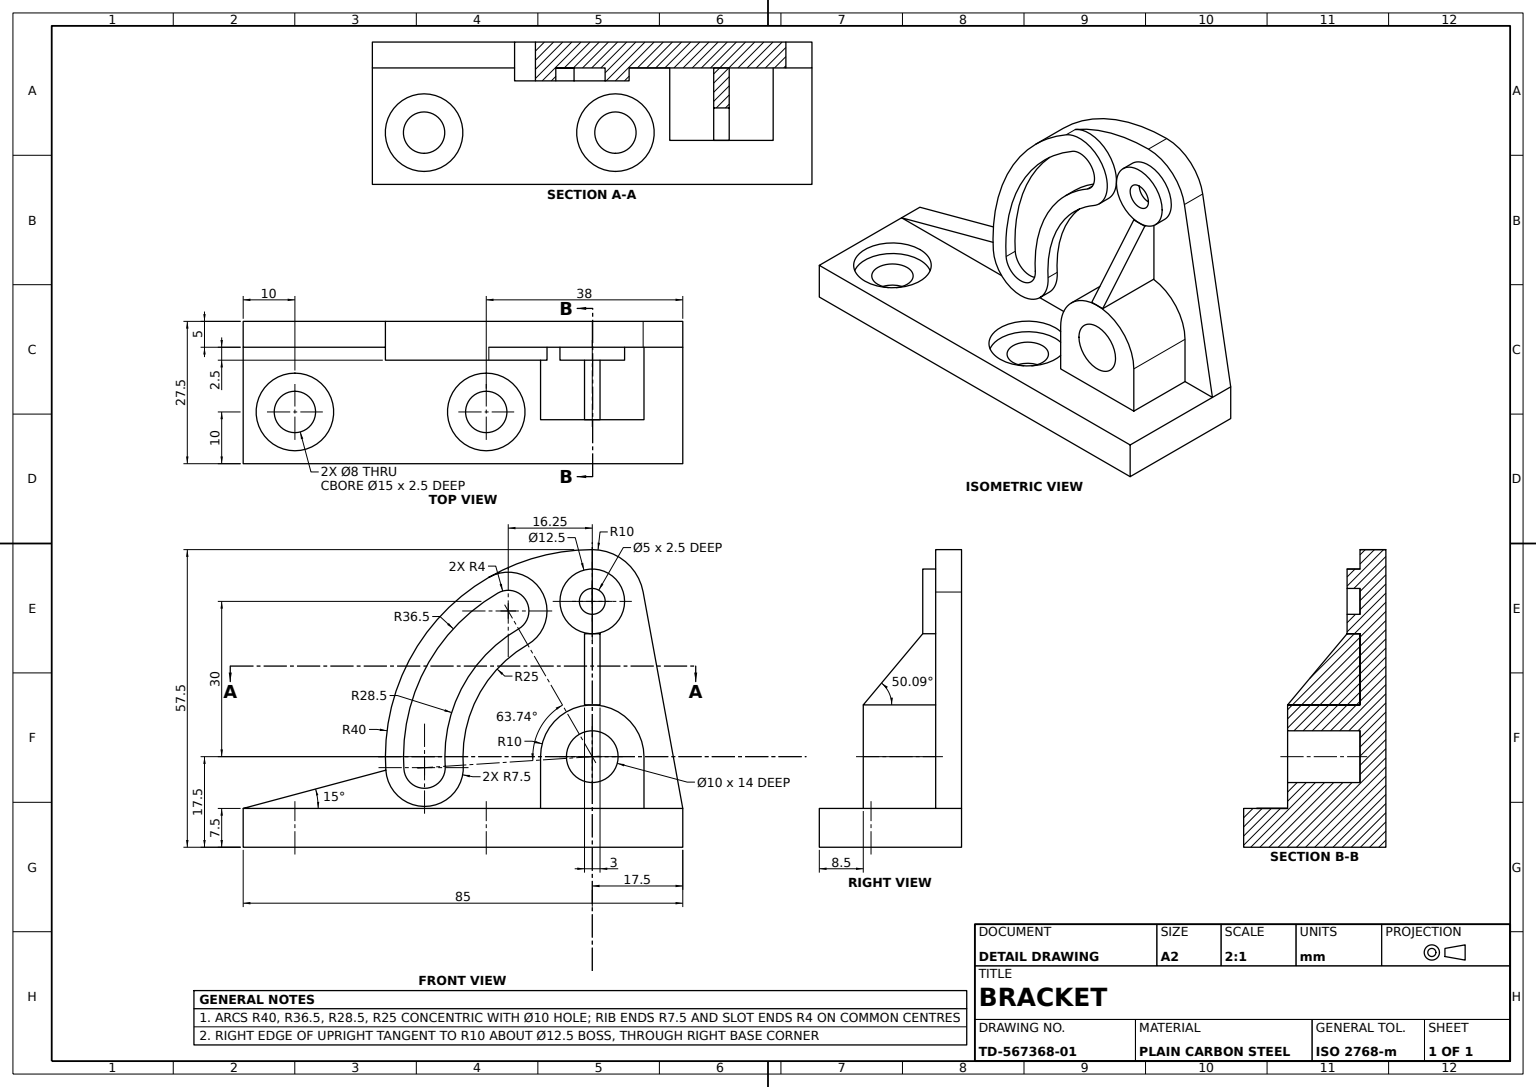
from build123d import *

# Parameters (mm, degrees)
BASE_PLATE_SKETCH_W         = 85
BASE_PLATE_SKETCH_H         = 27.5
BASE_PLATE_DEPTH            = 7.5
UPRIGHT_DEPTH               = 5
UPRIGHT_RIM_BOSS_SKETCH_R   = 6.25
UPRIGHT_RIM_BOSS_SKETCH_R_2 = 2.5
UPRIGHT_RIM_BOSS_DEPTH      = 2.5
BUSHING_BLOCK_SKETCH_R      = 5
BUSHING_BLOCK_DEPTH         = 14
COUNTERBORE_SKETCH_2X_15_R  = 7.5
COUNTERBORES_2X_15_DEPTH    = 2.5
MOUNTING_HOLE_SKETCH_2X_8_R = 4
MOUNTING_HOLES_2X_8_DEPTH   = 69.931578395
LINK_PLATE_DEPTH            = 1.5
CURVED_GUIDE_RIB_DEPTH      = 2.5


with BuildPart() as part:
    # Base Plate Sketch → Base Plate (new body)
    with BuildSketch(Plane(origin=(0, 0, 0), x_dir=(1, 0, 0), z_dir=(0, 1, 0))):
        Rectangle(BASE_PLATE_SKETCH_W, BASE_PLATE_SKETCH_H)
    extrude(amount=BASE_PLATE_DEPTH)

    # Upright Profile Sketch → Upright (add)
    with BuildSketch(Plane(origin=(0, 0, -13.75), x_dir=(-1, 0, 0), z_dir=(0, 0, -1))):
        with BuildLine():
            Line((42.5, 7.5), (14.914850651, 14.891418491))
            ThreePointArc((14.914850651, 14.891418491), (4.191978867, 44.846450772), (-25, 57.5))
            ThreePointArc((-25, 57.5), (-31.401843997, 55.182212796), (-34.836065574, 49.303278689))
            Line((-34.836065574, 49.303278689), (-42.5, 7.5))
            Line((-42.5, 7.5), (42.5, 7.5))
        make_face()
    extrude(amount=-UPRIGHT_DEPTH)

    # Upright Rim Boss Sketch → Upright Rim Boss (add)
    with BuildSketch(Plane.XY.offset(-8.75)):
        with Locations((25, 47.5)):
            Circle(UPRIGHT_RIM_BOSS_SKETCH_R)
        with Locations((25, 47.5)):
            Circle(UPRIGHT_RIM_BOSS_SKETCH_R_2, mode=Mode.SUBTRACT)
    extrude(amount=UPRIGHT_RIM_BOSS_DEPTH)

    # Bushing Block Sketch → Bushing Block (add)
    with BuildSketch(Plane.XY.offset(-8.75)):
        with BuildLine():
            Line((15, 17.5), (15, 7.5))
            Line((15, 7.5), (35, 7.5))
            Line((35, 7.5), (35, 17.5))
            ThreePointArc((35, 17.5), (25, 27.5), (15, 17.5))
        make_face()
        with Locations((25, 17.5)):
            Circle(BUSHING_BLOCK_SKETCH_R, mode=Mode.SUBTRACT)
    extrude(amount=BUSHING_BLOCK_DEPTH)

    # Counterbore Sketch 2xØ15 → Counterbores 2xØ15 (cut)
    with BuildSketch(Plane(origin=(0, 7.5, 0), x_dir=(1, 0, 0), z_dir=(0, 1, 0))):
        with Locations(Location((4.5, -3.75, 0), (0, 0, 270))):
            Circle(COUNTERBORE_SKETCH_2X_15_R)
        with Locations(Location((-32.5, -3.75, 0), (0, 0, 270))):
            Circle(COUNTERBORE_SKETCH_2X_15_R)
    extrude(amount=-COUNTERBORES_2X_15_DEPTH, mode=Mode.SUBTRACT)

    # Mounting Hole Sketch 2xØ8 → Mounting Holes 2xØ8 (cut, through all)
    with BuildSketch(Plane(origin=(0, 5, 0), x_dir=(1, 0, 0), z_dir=(0, 1, 0))):
        with Locations(Location((-32.5, -3.75, 0), (0, 0, 270))):
            Circle(MOUNTING_HOLE_SKETCH_2X_8_R)
        with Locations(Location((4.5, -3.75, 0), (0, 0, 270))):
            Circle(MOUNTING_HOLE_SKETCH_2X_8_R)
    extrude(amount=-MOUNTING_HOLES_2X_8_DEPTH, mode=Mode.SUBTRACT)

    # Curved Guide Rib Sketch → Curved Guide Rib (add)
    with BuildSketch(Plane.XY.offset(-8.75)):
        with BuildLine():
            ThreePointArc((5, 52.141016151), (-10.275068584, 36.359202963), (-14.914850651, 14.891418491))
            ThreePointArc((-14.914850651, 14.891418491), (-6.941707121, 7.896493027), (0.053218343, 15.869636557))
            ThreePointArc((0.053218343, 15.869636557), (2.953082135, 29.287001852), (12.5, 39.150635095))
            ThreePointArc((12.5, 39.150635095), (15.245190528, 49.395825623), (5, 52.141016151))
        make_face()
        with BuildLine():
            ThreePointArc((6.75, 49.109927238), (-7.188500083, 34.709022704), (-11.422301219, 15.119669373))
            ThreePointArc((-11.422301219, 15.119669373), (-7.169958003, 11.389042459), (-3.439331089, 15.641385675))
            ThreePointArc((-3.439331089, 15.641385675), (-0.133486366, 30.937182111), (10.75, 42.181724008))
            ThreePointArc((10.75, 42.181724008), (12.214101615, 47.645825623), (6.75, 49.109927238))
        make_face(mode=Mode.SUBTRACT)
    extrude(amount=CURVED_GUIDE_RIB_DEPTH)


with BuildPart() as body_2:
    # Link Plate Sketch → Link Plate (new, symmetric)
    with BuildSketch(Plane(origin=(25, 0, 0), x_dir=(0, 0, -1), z_dir=(1, 0, 0))):
        Polygon((6.25, 41.25), (-5.25, 27.5), (8.75, 27.5), (8.75, 41.25), align=None)
    extrude(amount=LINK_PLATE_DEPTH, both=True)


solid = Compound([part.part, body_2.part])
